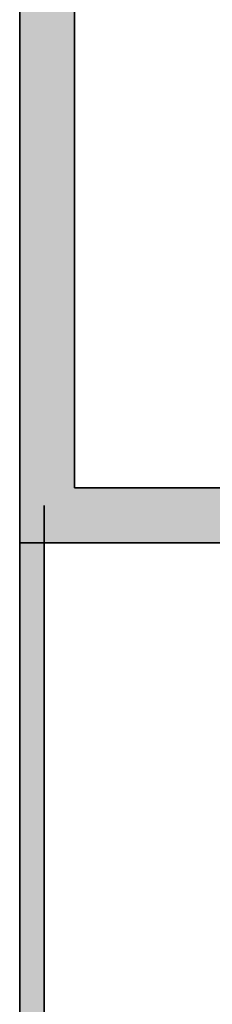
# Model space of a CAD drawing. Units: inches. Extents: x 1998 to 2588, y 1139 to 1977.
# Tile 7 of 134: x 2059 to 2075, y 1665 to 1746. Entities that reach past the tile are written whole.
import ezdxf

# ---------------------------------------------------------------- set-up
doc = ezdxf.new("R2010")
doc.units = ezdxf.units.IN
doc.layers.add('A-WALL-PATT', color=252, linetype='Continuous', lineweight=13)
doc.layers.add('WALL', color=200, linetype='Continuous', lineweight=35)

msp = doc.modelspace()

# ---------------------------------------------------------------- hatches: boundary and pattern name
at = {"layer": 'A-WALL-PATT'}
h = msp.add_hatch(color=256, dxfattribs=at)
h.dxf.hatch_style = 1
h.paths.add_polyline_path([(2227.4729, 1911.2324), (2222.9729, 1911.2324), (2222.9729, 1888.7324), (2227.4729, 1888.7324)])
h.paths.add_polyline_path([(2236.4493, 1870.3636), (2236.4493, 1875.2324), (2234.4125, 1875.2324), (2234.4125, 1868.3278), (2227.4729, 1868.3278), (2227.4729, 1866.2324), (2236.4493, 1866.2324)])
h.paths.add_polyline_path([(2330.0332, 1875.2324), (2263.9907, 1875.2324), (2263.9907, 1866.2324), (2330.0332, 1866.2324)])
h.paths.add_polyline_path([(2345.9729, 1906.7324), (2393.9729, 1906.7324), (2393.9729, 1882.7324), (2345.9729, 1882.7324), (2345.9729, 1878.2324), (2393.9729, 1878.2324), (2398.4729, 1878.2324), (2398.4729, 1882.7324), (2398.4729, 1911.2324), (2345.9729, 1911.2324), (2341.4729, 1911.2324), (2341.4729, 1866.2324), (2341.4729, 1790.0412), (2345.9729, 1790.0412), (2345.9729, 1875.2324)])
h.paths.add_polyline_path([(2398.4729, 1878.2324), (2393.9729, 1878.2324), (2393.9729, 1798.2324), (2393.9729, 1793.7324), (2398.4729, 1793.7324)], flags=17)
h.paths.add_polyline_path([(2393.9729, 1798.2324), (2375.7311, 1798.2324, -0.005968), (2375.7384, 1797.6146), (2375.7384, 1793.7324), (2393.9729, 1793.7324)], flags=17)
h.paths.add_polyline_path([(2349.8569, 1797.6146), (2349.8569, 1798.2324), (2345.9729, 1798.2324), (2345.9729, 1793.7324), (2349.8569, 1793.7324)], flags=17)
h.paths.add_polyline_path([(2398.4729, 1793.7324), (2393.9729, 1793.7324), (2393.9729, 1790.0412), (2398.4729, 1790.0412)], flags=17)
h.paths.add_polyline_path([(2527.4729, 1882.7324), (2507.8006, 1882.7324), (2507.8006, 1878.2324), (2518.4729, 1878.2324), (2518.4729, 1759.7324), (2510.9729, 1759.7324), (2510.9729, 1755.2324), (2527.4729, 1755.2324)])
h.paths.add_polyline_path([(2487.396, 1882.7324), (2398.4729, 1882.7324), (2398.4729, 1878.2324), (2487.396, 1878.2324)])
h.paths.add_polyline_path([(2490.5682, 1759.7324), (2345.9729, 1759.7324), (2345.9729, 1755.2324), (2490.5682, 1755.2324)])
h.paths.add_polyline_path([(2398.4729, 1760.5844), (2398.3914, 1760.5844), (2393.9729, 1760.5844), (2393.9729, 1759.7324), (2398.4729, 1759.7324)])
h.paths.add_polyline_path([(2334.5332, 1759.7324), (2234.4125, 1759.7324), (2234.4125, 1755.2324), (2334.5332, 1755.2324)])
h.paths.add_polyline_path([(2345.9729, 1760.5844), (2341.5543, 1760.5844), (2341.4729, 1760.5844), (2341.4729, 1759.7324), (2345.9729, 1759.7324)])
h.paths.add_polyline_path([(2222.9729, 1759.7324), (2221.7204, 1759.7324), (2221.7204, 1755.2324), (2222.9729, 1755.2324)])
h.paths.add_polyline_path([(2061.4729, 1702.7324), (2059.4729, 1702.7324), (2059.4729, 1584.2324), (2061.4729, 1584.2324)])
h.paths.add_polyline_path([(2061.4729, 1584.2324), (2059.4729, 1584.2324), (2059.4729, 1470.2324), (2061.4729, 1470.2324)])
h.paths.add_polyline_path([(2510.9729, 1469.2927), (2501.9729, 1469.2927), (2501.9729, 1369.172), (2510.9729, 1369.172)])
h.paths.add_polyline_path([(2227.4729, 1369.7324), (2227.4729, 1417.7324), (2221.4126, 1417.7324), (2221.4126, 1413.2324), (2222.9729, 1413.2324), (2222.9729, 1293.2324), (2222.9729, 1285.137), (2227.4729, 1285.137)])
h = msp.add_hatch(color=256, dxfattribs=at)
h.dxf.hatch_style = 1
h.paths.add_polyline_path([(2222.9729, 1888.7324), (2099.4125, 1888.7324), (2099.4125, 1879.7324), (2222.9729, 1879.7324)])
h.paths.add_polyline_path([(2096.9729, 1868.3278), (2087.9729, 1868.3278), (2087.9729, 1775.637), (2096.9729, 1775.637)])
h.paths.add_polyline_path([(2227.4729, 1868.3278), (2222.9729, 1868.3278), (2222.9729, 1774.3318), (2227.4729, 1774.3318)])
h.paths.add_polyline_path([(2188.3019, 1759.7324), (2138.6074, 1759.7324), (2099.4125, 1759.7324), (2099.4125, 1755.2324), (2176.9729, 1755.2324), (2188.3019, 1755.2324)])
h.paths.add_polyline_path([(2087.9729, 1759.7324), (2059.4729, 1759.7324), (2059.4729, 1702.7324), (2087.9729, 1702.7324), (2087.9729, 1707.2324), (2063.9729, 1707.2324), (2063.9729, 1755.2324), (2087.9729, 1755.2324)])
h.paths.add_polyline_path([(2096.9729, 1755.2324), (2087.9729, 1755.2324), (2087.9729, 1707.2324), (2096.9729, 1707.2324)])
h.paths.add_polyline_path([(2187.0461, 1707.2324), (2105.9729, 1707.2324), (2096.9729, 1707.2324), (2087.9729, 1707.2324), (2087.9729, 1702.7324), (2105.9729, 1702.7324), (2114.9729, 1702.7324), (2187.0461, 1702.7324)])
h.paths.add_polyline_path([(2181.4729, 1719.2028), (2176.9729, 1719.2028), (2176.9729, 1707.2324), (2181.4729, 1707.2324)])
h.paths.add_polyline_path([(2216.0332, 1588.7324), (2114.9729, 1588.7324), (2105.9729, 1588.7324), (2105.9729, 1584.2324), (2216.0332, 1584.2324)])
h.paths.add_polyline_path([(2077.691, 1588.7324), (2061.4729, 1588.7324), (2061.4729, 1584.2324), (2077.691, 1584.2324)])
h.paths.add_polyline_path([(2105.9729, 1588.7324), (2098.0956, 1588.7324), (2098.0956, 1584.2324), (2105.9729, 1584.2324)])
h.paths.add_polyline_path([(2114.9729, 1596.2642), (2110.1012, 1596.2642), (2105.9729, 1596.2642), (2105.9729, 1588.7324), (2114.9729, 1588.7324)])
h.paths.add_polyline_path([(2114.9729, 1584.2324), (2105.9729, 1584.2324), (2105.9729, 1580.249), (2110.1012, 1580.249), (2114.9729, 1580.249)])
h.paths.add_polyline_path([(2114.9729, 1547.7716), (2110.1012, 1547.7716, -0.0318759), (2105.9729, 1548.035), (2105.9729, 1470.2324), (2108.3775, 1470.2324), (2108.3775, 1465.7324), (2186.2943, 1465.7324), (2186.2943, 1470.2324), (2114.9729, 1470.2324)])
h.paths.add_polyline_path([(2227.4729, 1584.2324), (2222.9729, 1584.2324), (2222.9729, 1486.137), (2227.4729, 1486.137)])
h.paths.add_polyline_path([(2295.4138, 1593.2324), (2227.4729, 1593.2324), (2227.4729, 1588.7324), (2295.4138, 1588.7324), (2295.4138, 1591.8729)])
h.paths.add_polyline_path([(2345.9729, 1627.1165), (2341.4729, 1627.1165), (2341.4729, 1593.2324), (2337.2869, 1593.2324), (2337.2869, 1591.8729), (2337.2869, 1588.7324), (2345.9729, 1588.7324)])
h.paths.add_polyline_path([(2291.9729, 1588.7324), (2287.4729, 1588.7324), (2287.4729, 1522.7324), (2291.9729, 1522.7324)])
h.paths.add_polyline_path([(2291.9729, 1522.7324), (2287.4729, 1522.7324), (2227.4729, 1522.7324), (2227.4729, 1518.2324), (2291.9729, 1518.2324)])
h.paths.add_polyline_path([(2295.7347, 1519.5919), (2295.7347, 1522.7324), (2291.9729, 1522.7324), (2291.9729, 1518.2324), (2295.7347, 1518.2324)])
h.paths.add_polyline_path([(2345.9729, 1522.7324), (2337.6078, 1522.7324), (2337.6078, 1519.5919), (2337.6078, 1518.2324), (2341.4729, 1518.2324), (2341.4729, 1488.5616), (2345.9729, 1488.5616)])
h.paths.add_polyline_path([(2345.9729, 1468.1569), (2341.4729, 1468.1569), (2341.4729, 1374.2324), (2227.4729, 1374.2324), (2227.4729, 1369.7324), (2345.9729, 1369.7324)])
h.paths.add_polyline_path([(2345.9729, 1369.7324), (2341.4729, 1369.7324), (2341.4729, 1362.2324), (2345.9729, 1362.2324)])
h.paths.add_polyline_path([(2345.9729, 1317.7324), (2345.9729, 1322.2324), (2341.4729, 1322.2324), (2341.4729, 1285.137), (2345.9729, 1285.137)], flags=17)
h.paths.add_polyline_path([(2356.2096, 1322.2324), (2345.9729, 1322.2324), (2345.9729, 1317.7324), (2356.2096, 1317.7324), (2356.2096, 1319.3088)], flags=17)
h.paths.add_polyline_path([(2393.9729, 1322.2324), (2375.6999, 1322.2324), (2375.6999, 1319.3088, -0.0202458), (2375.636, 1317.7324), (2393.9729, 1317.7324)], flags=17)
h.paths.add_polyline_path([(2398.4729, 1322.2324), (2393.9729, 1322.2324), (2393.9729, 1317.7324), (2393.9729, 1237.7324), (2345.9729, 1237.7324), (2345.9729, 1264.7324), (2341.4729, 1264.7324), (2341.4729, 1228.7324), (2393.9729, 1228.7324), (2482.7412, 1228.7324), (2482.7412, 1237.7324), (2398.4729, 1237.7324), (2398.4729, 1297.1029)])
h.paths.add_polyline_path([(2398.4729, 1362.2324), (2393.9729, 1362.2324), (2393.9729, 1357.7324), (2398.4729, 1357.7324)])
h.paths.add_polyline_path([(2345.9729, 1329.7549), (2341.4729, 1329.7549), (2341.4729, 1322.2324), (2345.9729, 1322.2324)])

# ---------------------------------------------------------------- linework, layer by layer
at = {"layer": 'WALL'}
for p, q in [((2059.4729, 1759.7324), (2059.4729, 1702.7324)), ((2063.9729, 1755.2324), (2063.9729, 1707.2324)), ((2063.9729, 1707.2324), (2087.9729, 1707.2324)), ((2061.4729, 1473.2749), (2061.4729, 1705.7749)), ((2059.4729, 1702.7324), (2087.9729, 1702.7324)), ((2059.4729, 1470.2324), (2059.4729, 1702.7324))]:
    msp.add_line(p, q, dxfattribs=at)
msp.add_lwpolyline([(2059.4729, 1584.2324), (2061.4729, 1584.2324), (2061.4729, 1702.7324), (2059.4729, 1702.7324)], close=True, dxfattribs=at)

doc.saveas('drawing.dxf')
